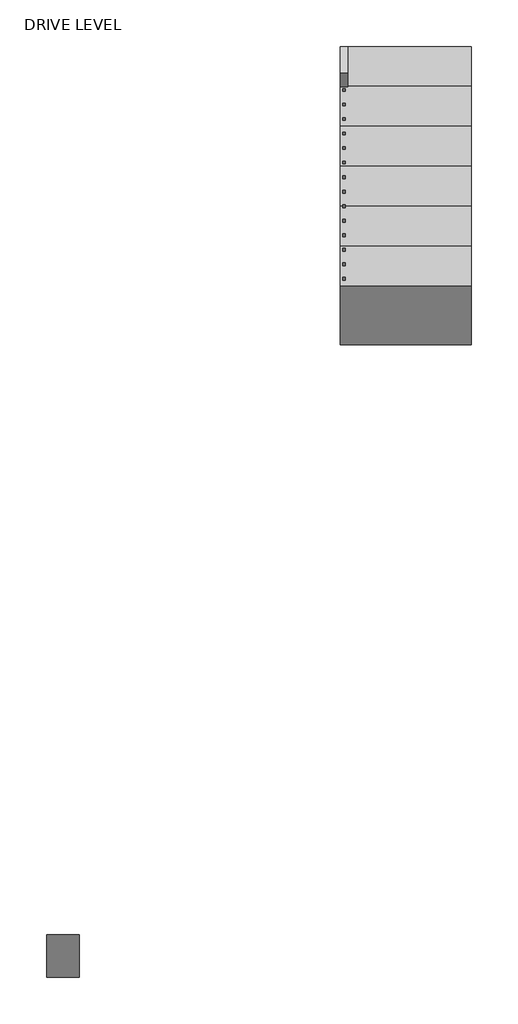
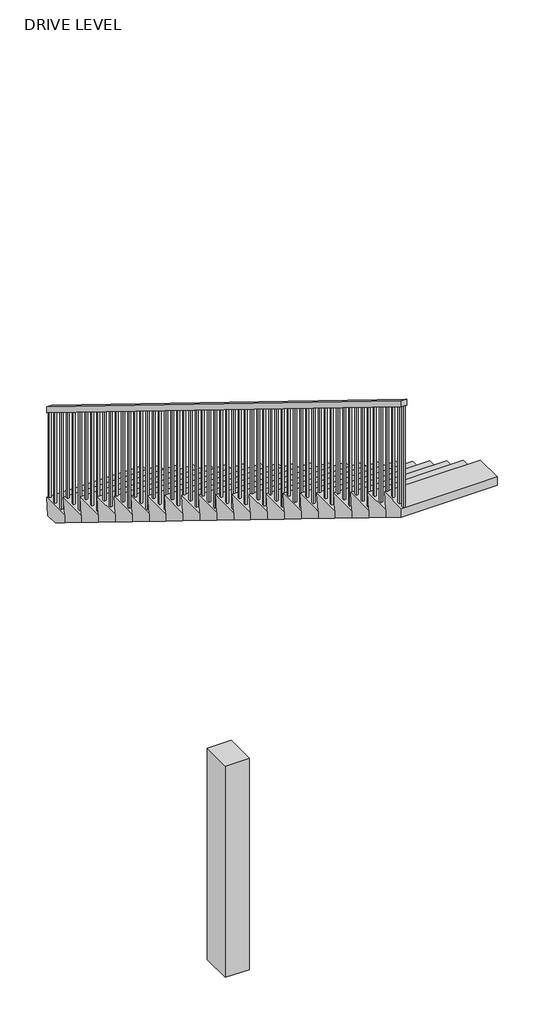
# One storey: 1 proxy, 1 railing, 1 stair flight.
"""IFC4 building model written with IfcOpenShell, lengths in millimetres."""

from ifc_helpers import new_model, si_unit, frame, origin, place, context, project, spatial, polyline, outline, extrude, faceted_brep, transform, mapped, element, save
from components import generic_models_1_generic_models_1_9fbe4478

model = new_model("IFC4")

# Units and contexts
model_context = context("Model", 3, world=origin())
ifc_project = project(units=[si_unit("LENGTHUNIT", "METRE", prefix="MILLI")], contexts=[model_context])

# Site, building, storey
site = spatial("IfcSite", under=ifc_project)
building = spatial("IfcBuilding", under=site)
storey = spatial("IfcBuildingStorey", under=building, Name="DRIVE LEVEL", Elevation=457.2)

# Proxy
placement = place(None, origin())
generic_models_1_generic_models_1_shape = generic_models_1_generic_models_1_9fbe4478(model_context)
element("IfcBuildingElementProxy", 1, Name="Generic Models 1 : Generic Models 1", ObjectType="Generic Models 1 : Generic Models 1", at=placement, inside=storey, context=model_context, shape_type="MappedRepresentation", body=[
    mapped(generic_models_1_generic_models_1_shape, transform((0.0, 0.0, 0.0), x_axis=(1.0, 0.0, 0.0), y_axis=(0.0, 1.0, 0.0), z_axis=(0.0, 0.0, 1.0))),
])

# Railing
element("IfcRailing", 2, ObjectType="Handrail - Rectangular", at=placement, inside=storey, context=model_context, shape_type="SweptSolid", body=[
    extrude(outline(polyline([(-5458.3521854, 1543.8782609), (-5458.3521854, 1484.1975237), (-11325.7521854, 5102.041002), (-11325.7521854, 5161.7217391), (-5458.3521854, 1543.8782609)])), frame((2204.5271331, 0.0, 0.0), z_axis=(1.0, 0.0, 0.0), x_axis=(0.0, 1.0, 0.0)), (0.0, 0.0, 1.0), 50.8),
    extrude(outline(polyline([(-11259.0771854, 5060.9291443), (-11240.0271854, 5049.1828992), (-11240.0271854, 4075.0434783), (-11259.0771854, 4075.0434783), (-11259.0771854, 5060.9291443)])), frame((2220.4021331, 0.0, 0.0), z_axis=(1.0, 0.0, 0.0), x_axis=(0.0, 1.0, 0.0)), (0.0, 0.0, 1.0), 19.05),
    extrude(outline(polyline([(-11157.4771854, 4998.282504), (-11138.4271854, 4986.5362589), (-11138.4271854, 4075.0434783), (-11157.4771854, 4075.0434783), (-11157.4771854, 4998.282504)])), frame((2220.4021331, 0.0, 0.0), z_axis=(1.0, 0.0, 0.0), x_axis=(0.0, 1.0, 0.0)), (0.0, 0.0, 1.0), 19.05),
    extrude(outline(polyline([(-11055.8771854, 4935.6358636), (-11036.8271854, 4923.8896186), (-11036.8271854, 4075.0434783), (-11055.8771854, 4075.0434783), (-11055.8771854, 4935.6358636)])), frame((2220.4021331, 0.0, 0.0), z_axis=(1.0, 0.0, 0.0), x_axis=(0.0, 1.0, 0.0)), (0.0, 0.0, 1.0), 19.05),
    extrude(outline(polyline([(-10954.2771854, 4872.9892233), (-10935.2271854, 4861.2429783), (-10935.2271854, 3902.7652174), (-10954.2771854, 3902.7652174), (-10954.2771854, 4872.9892233)])), frame((2220.4021331, 0.0, 0.0), z_axis=(1.0, 0.0, 0.0), x_axis=(0.0, 1.0, 0.0)), (0.0, 0.0, 1.0), 19.05),
    extrude(outline(polyline([(-10852.6771854, 4810.342583), (-10833.6271854, 4798.596338), (-10833.6271854, 3902.7652174), (-10852.6771854, 3902.7652174), (-10852.6771854, 4810.342583)])), frame((2220.4021331, 0.0, 0.0), z_axis=(1.0, 0.0, 0.0), x_axis=(0.0, 1.0, 0.0)), (0.0, 0.0, 1.0), 19.05),
    extrude(outline(polyline([(-10751.0771854, 4747.6959427), (-10732.0271854, 4735.9496976), (-10732.0271854, 3730.4869565), (-10751.0771854, 3730.4869565), (-10751.0771854, 4747.6959427)])), frame((2220.4021331, 0.0, 0.0), z_axis=(1.0, 0.0, 0.0), x_axis=(0.0, 1.0, 0.0)), (0.0, 0.0, 1.0), 19.05),
    extrude(outline(polyline([(-10649.4771854, 4685.0493024), (-10630.4271854, 4673.3030573), (-10630.4271854, 3730.4869565), (-10649.4771854, 3730.4869565), (-10649.4771854, 4685.0493024)])), frame((2220.4021331, 0.0, 0.0), z_axis=(1.0, 0.0, 0.0), x_axis=(0.0, 1.0, 0.0)), (0.0, 0.0, 1.0), 19.05),
    extrude(outline(polyline([(-10547.8771854, 4622.4026621), (-10528.8271854, 4610.656417), (-10528.8271854, 3730.4869565), (-10547.8771854, 3730.4869565), (-10547.8771854, 4622.4026621)])), frame((2220.4021331, 0.0, 0.0), z_axis=(1.0, 0.0, 0.0), x_axis=(0.0, 1.0, 0.0)), (0.0, 0.0, 1.0), 19.05),
    extrude(outline(polyline([(-10446.2771854, 4559.7560218), (-10427.2271854, 4548.0097767), (-10427.2271854, 3558.2086957), (-10446.2771854, 3558.2086957), (-10446.2771854, 4559.7560218)])), frame((2220.4021331, 0.0, 0.0), z_axis=(1.0, 0.0, 0.0), x_axis=(0.0, 1.0, 0.0)), (0.0, 0.0, 1.0), 19.05),
    extrude(outline(polyline([(-10344.6771854, 4497.1093814), (-10325.6271854, 4485.3631364), (-10325.6271854, 3558.2086957), (-10344.6771854, 3558.2086957), (-10344.6771854, 4497.1093814)])), frame((2220.4021331, 0.0, 0.0), z_axis=(1.0, 0.0, 0.0), x_axis=(0.0, 1.0, 0.0)), (0.0, 0.0, 1.0), 19.05),
    extrude(outline(polyline([(-10243.0771854, 4434.4627411), (-10224.0271854, 4422.7164961), (-10224.0271854, 3558.2086957), (-10243.0771854, 3558.2086957), (-10243.0771854, 4434.4627411)])), frame((2220.4021331, 0.0, 0.0), z_axis=(1.0, 0.0, 0.0), x_axis=(0.0, 1.0, 0.0)), (0.0, 0.0, 1.0), 19.05),
    extrude(outline(polyline([(-10141.4771854, 4371.8161008), (-10122.4271854, 4360.0698557), (-10122.4271854, 3385.9304348), (-10141.4771854, 3385.9304348), (-10141.4771854, 4371.8161008)])), frame((2220.4021331, 0.0, 0.0), z_axis=(1.0, 0.0, 0.0), x_axis=(0.0, 1.0, 0.0)), (0.0, 0.0, 1.0), 19.05),
    extrude(outline(polyline([(-10039.8771854, 4309.1694605), (-10020.8271854, 4297.4232154), (-10020.8271854, 3385.9304348), (-10039.8771854, 3385.9304348), (-10039.8771854, 4309.1694605)])), frame((2220.4021331, 0.0, 0.0), z_axis=(1.0, 0.0, 0.0), x_axis=(0.0, 1.0, 0.0)), (0.0, 0.0, 1.0), 19.05),
    extrude(outline(polyline([(-9938.2771854, 4246.5228202), (-9919.2271854, 4234.7765751), (-9919.2271854, 3385.9304348), (-9938.2771854, 3385.9304348), (-9938.2771854, 4246.5228202)])), frame((2220.4021331, 0.0, 0.0), z_axis=(1.0, 0.0, 0.0), x_axis=(0.0, 1.0, 0.0)), (0.0, 0.0, 1.0), 19.05),
    extrude(outline(polyline([(-9836.6771854, 4183.8761799), (-9817.6271854, 4172.1299348), (-9817.6271854, 3213.6521739), (-9836.6771854, 3213.6521739), (-9836.6771854, 4183.8761799)])), frame((2220.4021331, 0.0, 0.0), z_axis=(1.0, 0.0, 0.0), x_axis=(0.0, 1.0, 0.0)), (0.0, 0.0, 1.0), 19.05),
    extrude(outline(polyline([(-9735.0771854, 4121.2295395), (-9716.0271854, 4109.4832945), (-9716.0271854, 3213.6521739), (-9735.0771854, 3213.6521739), (-9735.0771854, 4121.2295395)])), frame((2220.4021331, 0.0, 0.0), z_axis=(1.0, 0.0, 0.0), x_axis=(0.0, 1.0, 0.0)), (0.0, 0.0, 1.0), 19.05),
    extrude(outline(polyline([(-9633.4771854, 4058.5828992), (-9614.4271854, 4046.8366542), (-9614.4271854, 3041.373913), (-9633.4771854, 3041.373913), (-9633.4771854, 4058.5828992)])), frame((2220.4021331, 0.0, 0.0), z_axis=(1.0, 0.0, 0.0), x_axis=(0.0, 1.0, 0.0)), (0.0, 0.0, 1.0), 19.05),
    extrude(outline(polyline([(-9531.8771854, 3995.9362589), (-9512.8271854, 3984.1900138), (-9512.8271854, 3041.373913), (-9531.8771854, 3041.373913), (-9531.8771854, 3995.9362589)])), frame((2220.4021331, 0.0, 0.0), z_axis=(1.0, 0.0, 0.0), x_axis=(0.0, 1.0, 0.0)), (0.0, 0.0, 1.0), 19.05),
    extrude(outline(polyline([(-9430.2771854, 3933.2896186), (-9411.2271854, 3921.5433735), (-9411.2271854, 3041.373913), (-9430.2771854, 3041.373913), (-9430.2771854, 3933.2896186)])), frame((2220.4021331, 0.0, 0.0), z_axis=(1.0, 0.0, 0.0), x_axis=(0.0, 1.0, 0.0)), (0.0, 0.0, 1.0), 19.05),
    extrude(outline(polyline([(-9328.6771854, 3870.6429783), (-9309.6271854, 3858.8967332), (-9309.6271854, 2869.0956522), (-9328.6771854, 2869.0956522), (-9328.6771854, 3870.6429783)])), frame((2220.4021331, 0.0, 0.0), z_axis=(1.0, 0.0, 0.0), x_axis=(0.0, 1.0, 0.0)), (0.0, 0.0, 1.0), 19.05),
    extrude(outline(polyline([(-9227.0771854, 3807.996338), (-9208.0271854, 3796.2500929), (-9208.0271854, 2869.0956522), (-9227.0771854, 2869.0956522), (-9227.0771854, 3807.996338)])), frame((2220.4021331, 0.0, 0.0), z_axis=(1.0, 0.0, 0.0), x_axis=(0.0, 1.0, 0.0)), (0.0, 0.0, 1.0), 19.05),
    extrude(outline(polyline([(-9125.4771854, 3745.3496976), (-9106.4271854, 3733.6034526), (-9106.4271854, 2869.0956522), (-9125.4771854, 2869.0956522), (-9125.4771854, 3745.3496976)])), frame((2220.4021331, 0.0, 0.0), z_axis=(1.0, 0.0, 0.0), x_axis=(0.0, 1.0, 0.0)), (0.0, 0.0, 1.0), 19.05),
    extrude(outline(polyline([(-9023.8771854, 3682.7030573), (-9004.8271854, 3670.9568123), (-9004.8271854, 2696.8173913), (-9023.8771854, 2696.8173913), (-9023.8771854, 3682.7030573)])), frame((2220.4021331, 0.0, 0.0), z_axis=(1.0, 0.0, 0.0), x_axis=(0.0, 1.0, 0.0)), (0.0, 0.0, 1.0), 19.05),
    extrude(outline(polyline([(-8922.2771854, 3620.056417), (-8903.2271854, 3608.3101719), (-8903.2271854, 2696.8173913), (-8922.2771854, 2696.8173913), (-8922.2771854, 3620.056417)])), frame((2220.4021331, 0.0, 0.0), z_axis=(1.0, 0.0, 0.0), x_axis=(0.0, 1.0, 0.0)), (0.0, 0.0, 1.0), 19.05),
    extrude(outline(polyline([(-8820.6771854, 3557.4097767), (-8801.6271854, 3545.6635316), (-8801.6271854, 2696.8173913), (-8820.6771854, 2696.8173913), (-8820.6771854, 3557.4097767)])), frame((2220.4021331, 0.0, 0.0), z_axis=(1.0, 0.0, 0.0), x_axis=(0.0, 1.0, 0.0)), (0.0, 0.0, 1.0), 19.05),
    extrude(outline(polyline([(-8719.0771854, 3494.7631364), (-8700.0271854, 3483.0168913), (-8700.0271854, 2524.5391304), (-8719.0771854, 2524.5391304), (-8719.0771854, 3494.7631364)])), frame((2220.4021331, 0.0, 0.0), z_axis=(1.0, 0.0, 0.0), x_axis=(0.0, 1.0, 0.0)), (0.0, 0.0, 1.0), 19.05),
    extrude(outline(polyline([(-8617.4771854, 3432.1164961), (-8598.4271854, 3420.370251), (-8598.4271854, 2524.5391304), (-8617.4771854, 2524.5391304), (-8617.4771854, 3432.1164961)])), frame((2220.4021331, 0.0, 0.0), z_axis=(1.0, 0.0, 0.0), x_axis=(0.0, 1.0, 0.0)), (0.0, 0.0, 1.0), 19.05),
    extrude(outline(polyline([(-8515.8771854, 3369.4698557), (-8496.8271854, 3357.7236107), (-8496.8271854, 2352.2608696), (-8515.8771854, 2352.2608696), (-8515.8771854, 3369.4698557)])), frame((2220.4021331, 0.0, 0.0), z_axis=(1.0, 0.0, 0.0), x_axis=(0.0, 1.0, 0.0)), (0.0, 0.0, 1.0), 19.05),
    extrude(outline(polyline([(-8414.2771854, 3306.8232154), (-8395.2271854, 3295.0769704), (-8395.2271854, 2352.2608696), (-8414.2771854, 2352.2608696), (-8414.2771854, 3306.8232154)])), frame((2220.4021331, 0.0, 0.0), z_axis=(1.0, 0.0, 0.0), x_axis=(0.0, 1.0, 0.0)), (0.0, 0.0, 1.0), 19.05),
    extrude(outline(polyline([(-8312.6771854, 3244.1765751), (-8293.6271854, 3232.4303301), (-8293.6271854, 2352.2608696), (-8312.6771854, 2352.2608696), (-8312.6771854, 3244.1765751)])), frame((2220.4021331, 0.0, 0.0), z_axis=(1.0, 0.0, 0.0), x_axis=(0.0, 1.0, 0.0)), (0.0, 0.0, 1.0), 19.05),
    extrude(outline(polyline([(-8211.0771854, 3181.5299348), (-8192.0271854, 3169.7836897), (-8192.0271854, 2179.9826087), (-8211.0771854, 2179.9826087), (-8211.0771854, 3181.5299348)])), frame((2220.4021331, 0.0, 0.0), z_axis=(1.0, 0.0, 0.0), x_axis=(0.0, 1.0, 0.0)), (0.0, 0.0, 1.0), 19.05),
    extrude(outline(polyline([(-8109.4771854, 3118.8832945), (-8090.4271854, 3107.1370494), (-8090.4271854, 2179.9826087), (-8109.4771854, 2179.9826087), (-8109.4771854, 3118.8832945)])), frame((2220.4021331, 0.0, 0.0), z_axis=(1.0, 0.0, 0.0), x_axis=(0.0, 1.0, 0.0)), (0.0, 0.0, 1.0), 19.05),
    extrude(outline(polyline([(-8007.8771854, 3056.2366542), (-7988.8271854, 3044.4904091), (-7988.8271854, 2179.9826087), (-8007.8771854, 2179.9826087), (-8007.8771854, 3056.2366542)])), frame((2220.4021331, 0.0, 0.0), z_axis=(1.0, 0.0, 0.0), x_axis=(0.0, 1.0, 0.0)), (0.0, 0.0, 1.0), 19.05),
    extrude(outline(polyline([(-7906.2771854, 2993.5900138), (-7887.2271854, 2981.8437688), (-7887.2271854, 2007.7043478), (-7906.2771854, 2007.7043478), (-7906.2771854, 2993.5900138)])), frame((2220.4021331, 0.0, 0.0), z_axis=(1.0, 0.0, 0.0), x_axis=(0.0, 1.0, 0.0)), (0.0, 0.0, 1.0), 19.05),
    extrude(outline(polyline([(-7804.6771854, 2930.9433735), (-7785.6271854, 2919.1971285), (-7785.6271854, 2007.7043478), (-7804.6771854, 2007.7043478), (-7804.6771854, 2930.9433735)])), frame((2220.4021331, 0.0, 0.0), z_axis=(1.0, 0.0, 0.0), x_axis=(0.0, 1.0, 0.0)), (0.0, 0.0, 1.0), 19.05),
    extrude(outline(polyline([(-7703.0771854, 2868.2967332), (-7684.0271854, 2856.5504882), (-7684.0271854, 2007.7043478), (-7703.0771854, 2007.7043478), (-7703.0771854, 2868.2967332)])), frame((2220.4021331, 0.0, 0.0), z_axis=(1.0, 0.0, 0.0), x_axis=(0.0, 1.0, 0.0)), (0.0, 0.0, 1.0), 19.05),
    extrude(outline(polyline([(-7601.4771854, 2805.6500929), (-7582.4271854, 2793.9038478), (-7582.4271854, 1835.426087), (-7601.4771854, 1835.426087), (-7601.4771854, 2805.6500929)])), frame((2220.4021331, 0.0, 0.0), z_axis=(1.0, 0.0, 0.0), x_axis=(0.0, 1.0, 0.0)), (0.0, 0.0, 1.0), 19.05),
    extrude(outline(polyline([(-7499.8771854, 2743.0034526), (-7480.8271854, 2731.2572075), (-7480.8271854, 1835.426087), (-7499.8771854, 1835.426087), (-7499.8771854, 2743.0034526)])), frame((2220.4021331, 0.0, 0.0), z_axis=(1.0, 0.0, 0.0), x_axis=(0.0, 1.0, 0.0)), (0.0, 0.0, 1.0), 19.05),
    extrude(outline(polyline([(-7398.2771854, 2680.3568123), (-7379.2271854, 2668.6105672), (-7379.2271854, 1663.1478261), (-7398.2771854, 1663.1478261), (-7398.2771854, 2680.3568123)])), frame((2220.4021331, 0.0, 0.0), z_axis=(1.0, 0.0, 0.0), x_axis=(0.0, 1.0, 0.0)), (0.0, 0.0, 1.0), 19.05),
    extrude(outline(polyline([(-7296.6771854, 2617.7101719), (-7277.6271854, 2605.9639269), (-7277.6271854, 1663.1478261), (-7296.6771854, 1663.1478261), (-7296.6771854, 2617.7101719)])), frame((2220.4021331, 0.0, 0.0), z_axis=(1.0, 0.0, 0.0), x_axis=(0.0, 1.0, 0.0)), (0.0, 0.0, 1.0), 19.05),
    extrude(outline(polyline([(-7195.0771854, 2555.0635316), (-7176.0271854, 2543.3172866), (-7176.0271854, 1663.1478261), (-7195.0771854, 1663.1478261), (-7195.0771854, 2555.0635316)])), frame((2220.4021331, 0.0, 0.0), z_axis=(1.0, 0.0, 0.0), x_axis=(0.0, 1.0, 0.0)), (0.0, 0.0, 1.0), 19.05),
    extrude(outline(polyline([(-7093.4771854, 2492.4168913), (-7074.4271854, 2480.6706463), (-7074.4271854, 1490.8695652), (-7093.4771854, 1490.8695652), (-7093.4771854, 2492.4168913)])), frame((2220.4021331, 0.0, 0.0), z_axis=(1.0, 0.0, 0.0), x_axis=(0.0, 1.0, 0.0)), (0.0, 0.0, 1.0), 19.05),
    extrude(outline(polyline([(-6991.8771854, 2429.770251), (-6972.8271854, 2418.0240059), (-6972.8271854, 1490.8695652), (-6991.8771854, 1490.8695652), (-6991.8771854, 2429.770251)])), frame((2220.4021331, 0.0, 0.0), z_axis=(1.0, 0.0, 0.0), x_axis=(0.0, 1.0, 0.0)), (0.0, 0.0, 1.0), 19.05),
    extrude(outline(polyline([(-6890.2771854, 2367.1236107), (-6871.2271854, 2355.3773656), (-6871.2271854, 1490.8695652), (-6890.2771854, 1490.8695652), (-6890.2771854, 2367.1236107)])), frame((2220.4021331, 0.0, 0.0), z_axis=(1.0, 0.0, 0.0), x_axis=(0.0, 1.0, 0.0)), (0.0, 0.0, 1.0), 19.05),
    extrude(outline(polyline([(-6788.6771854, 2304.4769704), (-6769.6271854, 2292.7307253), (-6769.6271854, 1318.5913043), (-6788.6771854, 1318.5913043), (-6788.6771854, 2304.4769704)])), frame((2220.4021331, 0.0, 0.0), z_axis=(1.0, 0.0, 0.0), x_axis=(0.0, 1.0, 0.0)), (0.0, 0.0, 1.0), 19.05),
    extrude(outline(polyline([(-6687.0771854, 2241.8303301), (-6668.0271854, 2230.084085), (-6668.0271854, 1318.5913043), (-6687.0771854, 1318.5913043), (-6687.0771854, 2241.8303301)])), frame((2220.4021331, 0.0, 0.0), z_axis=(1.0, 0.0, 0.0), x_axis=(0.0, 1.0, 0.0)), (0.0, 0.0, 1.0), 19.05),
    extrude(outline(polyline([(-6585.4771854, 2179.1836897), (-6566.4271854, 2167.4374447), (-6566.4271854, 1318.5913043), (-6585.4771854, 1318.5913043), (-6585.4771854, 2179.1836897)])), frame((2220.4021331, 0.0, 0.0), z_axis=(1.0, 0.0, 0.0), x_axis=(0.0, 1.0, 0.0)), (0.0, 0.0, 1.0), 19.05),
    extrude(outline(polyline([(-6483.8771854, 2116.5370494), (-6464.8271854, 2104.7908044), (-6464.8271854, 1146.3130435), (-6483.8771854, 1146.3130435), (-6483.8771854, 2116.5370494)])), frame((2220.4021331, 0.0, 0.0), z_axis=(1.0, 0.0, 0.0), x_axis=(0.0, 1.0, 0.0)), (0.0, 0.0, 1.0), 19.05),
    extrude(outline(polyline([(-6382.2771854, 2053.8904091), (-6363.2271854, 2042.144164), (-6363.2271854, 1146.3130435), (-6382.2771854, 1146.3130435), (-6382.2771854, 2053.8904091)])), frame((2220.4021331, 0.0, 0.0), z_axis=(1.0, 0.0, 0.0), x_axis=(0.0, 1.0, 0.0)), (0.0, 0.0, 1.0), 19.05),
    extrude(outline(polyline([(-6280.6771854, 1991.2437688), (-6261.6271854, 1979.4975237), (-6261.6271854, 974.0347826), (-6280.6771854, 974.0347826), (-6280.6771854, 1991.2437688)])), frame((2220.4021331, 0.0, 0.0), z_axis=(1.0, 0.0, 0.0), x_axis=(0.0, 1.0, 0.0)), (0.0, 0.0, 1.0), 19.05),
    extrude(outline(polyline([(-6179.0771854, 1928.5971285), (-6160.0271854, 1916.8508834), (-6160.0271854, 974.0347826), (-6179.0771854, 974.0347826), (-6179.0771854, 1928.5971285)])), frame((2220.4021331, 0.0, 0.0), z_axis=(1.0, 0.0, 0.0), x_axis=(0.0, 1.0, 0.0)), (0.0, 0.0, 1.0), 19.05),
    extrude(outline(polyline([(-6077.4771854, 1865.9504882), (-6058.4271854, 1854.2042431), (-6058.4271854, 974.0347826), (-6077.4771854, 974.0347826), (-6077.4771854, 1865.9504882)])), frame((2220.4021331, 0.0, 0.0), z_axis=(1.0, 0.0, 0.0), x_axis=(0.0, 1.0, 0.0)), (0.0, 0.0, 1.0), 19.05),
    extrude(outline(polyline([(-5975.8771854, 1803.3038478), (-5956.8271854, 1791.5576028), (-5956.8271854, 801.7565217), (-5975.8771854, 801.7565217), (-5975.8771854, 1803.3038478)])), frame((2220.4021331, 0.0, 0.0), z_axis=(1.0, 0.0, 0.0), x_axis=(0.0, 1.0, 0.0)), (0.0, 0.0, 1.0), 19.05),
    extrude(outline(polyline([(-5874.2771854, 1740.6572075), (-5855.2271854, 1728.9109625), (-5855.2271854, 801.7565217), (-5874.2771854, 801.7565217), (-5874.2771854, 1740.6572075)])), frame((2220.4021331, 0.0, 0.0), z_axis=(1.0, 0.0, 0.0), x_axis=(0.0, 1.0, 0.0)), (0.0, 0.0, 1.0), 19.05),
    extrude(outline(polyline([(-5772.6771854, 1678.0105672), (-5753.6271854, 1666.2643221), (-5753.6271854, 801.7565217), (-5772.6771854, 801.7565217), (-5772.6771854, 1678.0105672)])), frame((2220.4021331, 0.0, 0.0), z_axis=(1.0, 0.0, 0.0), x_axis=(0.0, 1.0, 0.0)), (0.0, 0.0, 1.0), 19.05),
    extrude(outline(polyline([(-5671.0771854, 1615.3639269), (-5652.0271854, 1603.6176818), (-5652.0271854, 629.4782609), (-5671.0771854, 629.4782609), (-5671.0771854, 1615.3639269)])), frame((2220.4021331, 0.0, 0.0), z_axis=(1.0, 0.0, 0.0), x_axis=(0.0, 1.0, 0.0)), (0.0, 0.0, 1.0), 19.05),
    extrude(outline(polyline([(-5569.4771854, 1552.7172866), (-5550.4271854, 1540.9710415), (-5550.4271854, 629.4782609), (-5569.4771854, 629.4782609), (-5569.4771854, 1552.7172866)])), frame((2220.4021331, 0.0, 0.0), z_axis=(1.0, 0.0, 0.0), x_axis=(0.0, 1.0, 0.0)), (0.0, 0.0, 1.0), 19.05),
    extrude(outline(polyline([(-11325.7521854, 5102.041002), (-11306.7021854, 5090.2947569), (-11306.7021854, 4075.0434783), (-11325.7521854, 4075.0434783), (-11325.7521854, 5102.041002)])), frame((2220.4021331, 0.0, 0.0), z_axis=(1.0, 0.0, 0.0), x_axis=(0.0, 1.0, 0.0)), (0.0, 0.0, 1.0), 19.05),
    extrude(outline(polyline([(-5477.4021854, 1495.9437688), (-5458.3521854, 1484.1975237), (-5458.3521854, 629.4782609), (-5477.4021854, 629.4782609), (-5477.4021854, 1495.9437688)])), frame((2220.4021331, 0.0, 0.0), z_axis=(1.0, 0.0, 0.0), x_axis=(0.0, 1.0, 0.0)), (0.0, 0.0, 1.0), 19.05),
])

# Stair flight
element("IfcStairFlight", 3, ObjectType="3/4\" Nosing", at=placement, inside=storey, context=model_context, shape_type="Brep", body=[
    faceted_brep([(3118.9271331, -5458.3521854, 629.4782609), (2204.5271331, -5458.3521854, 629.4782609), (2204.5271331, -5756.8021854, 629.4782609), (3118.9271331, -5756.8021854, 629.4782609), (3118.9271331, -5756.8021854, 554.8773394), (3118.9271331, -5598.3895772, 457.2), (3118.9271331, -5477.4021854, 457.2), (2204.5271331, -5477.4021854, 457.2), (2204.5271331, -5598.3895772, 457.2), (2204.5271331, -5756.8021854, 554.8773394), (3118.9271331, -5737.7521854, 801.7565217), (2204.5271331, -5737.7521854, 801.7565217), (2204.5271331, -6036.2021854, 801.7565217), (3118.9271331, -6036.2021854, 801.7565217), (3118.9271331, -6036.2021854, 727.1556003), (2204.5271331, -6036.2021854, 727.1556003), (3118.9271331, -6017.1521854, 974.0347826), (2204.5271331, -6017.1521854, 974.0347826), (2204.5271331, -6315.6021854, 974.0347826), (3118.9271331, -6315.6021854, 974.0347826), (3118.9271331, -6315.6021854, 899.4338612), (2204.5271331, -6315.6021854, 899.4338612), (3118.9271331, -6296.5521854, 1146.3130435), (2204.5271331, -6296.5521854, 1146.3130435), (2204.5271331, -6595.0021854, 1146.3130435), (3118.9271331, -6595.0021854, 1146.3130435), (3118.9271331, -6595.0021854, 1071.7121221), (2204.5271331, -6595.0021854, 1071.7121221), (3118.9271331, -6575.9521854, 1318.5913043), (2204.5271331, -6575.9521854, 1318.5913043), (2204.5271331, -6874.4021854, 1318.5913043), (3118.9271331, -6874.4021854, 1318.5913043), (3118.9271331, -6874.4021854, 1243.9903829), (2204.5271331, -6874.4021854, 1243.9903829), (3118.9271331, -6855.3521854, 1490.8695652), (2204.5271331, -6855.3521854, 1490.8695652), (2204.5271331, -7153.8021854, 1490.8695652), (3118.9271331, -7153.8021854, 1490.8695652), (3118.9271331, -7153.8021854, 1416.2686438), (2204.5271331, -7153.8021854, 1416.2686438), (3118.9271331, -7134.7521854, 1663.1478261), (2204.5271331, -7134.7521854, 1663.1478261), (2204.5271331, -7433.2021854, 1663.1478261), (3118.9271331, -7433.2021854, 1663.1478261), (3118.9271331, -7433.2021854, 1588.5469047), (2204.5271331, -7433.2021854, 1588.5469047), (3118.9271331, -7414.1521854, 1835.426087), (2204.5271331, -7414.1521854, 1835.426087), (2204.5271331, -7712.6021854, 1835.426087), (3118.9271331, -7712.6021854, 1835.426087), (3118.9271331, -7712.6021854, 1760.8251655), (2204.5271331, -7712.6021854, 1760.8251655), (3118.9271331, -7693.5521854, 2007.7043478), (2204.5271331, -7693.5521854, 2007.7043478), (2204.5271331, -7992.0021854, 2007.7043478), (3118.9271331, -7992.0021854, 2007.7043478), (3118.9271331, -7992.0021854, 1933.1034264), (2204.5271331, -7992.0021854, 1933.1034264), (3118.9271331, -7972.9521854, 2179.9826087), (2204.5271331, -7972.9521854, 2179.9826087), (2204.5271331, -8271.4021854, 2179.9826087), (3118.9271331, -8271.4021854, 2179.9826087), (3118.9271331, -8271.4021854, 2105.3816873), (2204.5271331, -8271.4021854, 2105.3816873), (3118.9271331, -8252.3521854, 2352.2608696), (2204.5271331, -8252.3521854, 2352.2608696), (2204.5271331, -8550.8021854, 2352.2608696), (3118.9271331, -8550.8021854, 2352.2608696), (3118.9271331, -8550.8021854, 2277.6599481), (2204.5271331, -8550.8021854, 2277.6599481), (3118.9271331, -8830.2021854, 2449.938209), (3118.9271331, -9109.6021854, 2622.2164699), (3118.9271331, -9389.0021854, 2794.4947307), (3118.9271331, -9668.4021854, 2966.7729916), (3118.9271331, -9947.8021854, 3139.0512525), (3118.9271331, -10227.2021854, 3311.3295134), (3118.9271331, -10506.6021854, 3483.6077742), (3118.9271331, -10786.0021854, 3655.8860351), (3118.9271331, -11065.4021854, 3828.164296), (3118.9271331, -11325.7521854, 3988.6963118), (2204.5271331, -11325.7521854, 3988.6963118), (2204.5271331, -11065.4021854, 3828.164296), (2204.5271331, -10786.0021854, 3655.8860351), (2204.5271331, -10506.6021854, 3483.6077742), (2204.5271331, -10227.2021854, 3311.3295134), (2204.5271331, -9947.8021854, 3139.0512525), (2204.5271331, -9668.4021854, 2966.7729916), (2204.5271331, -9389.0021854, 2794.4947307), (2204.5271331, -9109.6021854, 2622.2164699), (2204.5271331, -8830.2021854, 2449.938209), (3118.9271331, -8531.7521854, 2524.5391304), (2204.5271331, -8531.7521854, 2524.5391304), (2204.5271331, -8830.2021854, 2524.5391304), (3118.9271331, -8830.2021854, 2524.5391304), (3118.9271331, -8811.1521854, 2696.8173913), (2204.5271331, -8811.1521854, 2696.8173913), (2204.5271331, -9109.6021854, 2696.8173913), (3118.9271331, -9109.6021854, 2696.8173913), (3118.9271331, -9090.5521854, 2869.0956522), (2204.5271331, -9090.5521854, 2869.0956522), (2204.5271331, -9389.0021854, 2869.0956522), (3118.9271331, -9389.0021854, 2869.0956522), (3118.9271331, -9369.9521854, 3041.373913), (2204.5271331, -9369.9521854, 3041.373913), (2204.5271331, -9668.4021854, 3041.373913), (3118.9271331, -9668.4021854, 3041.373913), (3118.9271331, -9649.3521854, 3213.6521739), (2204.5271331, -9649.3521854, 3213.6521739), (2204.5271331, -9947.8021854, 3213.6521739), (3118.9271331, -9947.8021854, 3213.6521739), (3118.9271331, -9928.7521854, 3385.9304348), (2204.5271331, -9928.7521854, 3385.9304348), (2204.5271331, -10227.2021854, 3385.9304348), (3118.9271331, -10227.2021854, 3385.9304348), (3118.9271331, -10208.1521854, 3558.2086957), (2204.5271331, -10208.1521854, 3558.2086957), (2204.5271331, -10506.6021854, 3558.2086957), (3118.9271331, -10506.6021854, 3558.2086957), (3118.9271331, -10487.5521854, 3730.4869565), (2204.5271331, -10487.5521854, 3730.4869565), (2204.5271331, -10786.0021854, 3730.4869565), (3118.9271331, -10786.0021854, 3730.4869565), (3118.9271331, -10766.9521854, 3902.7652174), (2204.5271331, -10766.9521854, 3902.7652174), (2204.5271331, -11065.4021854, 3902.7652174), (3118.9271331, -11065.4021854, 3902.7652174), (3118.9271331, -11046.3521854, 4075.0434783), (2204.5271331, -11046.3521854, 4075.0434783), (2204.5271331, -11325.7521854, 4075.0434783), (3118.9271331, -11325.7521854, 4075.0434783)], [[[0, 1, 2, 3]], [[0, 3, 4, 5, 6]], [[2, 1, 7, 8, 9]], [[10, 11, 12, 13]], [[10, 13, 14, 4, 3]], [[12, 11, 2, 9, 15]], [[16, 17, 18, 19]], [[16, 19, 20, 14, 13]], [[18, 17, 12, 15, 21]], [[22, 23, 24, 25]], [[22, 25, 26, 20, 19]], [[24, 23, 18, 21, 27]], [[28, 29, 30, 31]], [[28, 31, 32, 26, 25]], [[30, 29, 24, 27, 33]], [[34, 35, 36, 37]], [[34, 37, 38, 32, 31]], [[36, 35, 30, 33, 39]], [[40, 41, 42, 43]], [[40, 43, 44, 38, 37]], [[42, 41, 36, 39, 45]], [[46, 47, 48, 49]], [[46, 49, 50, 44, 43]], [[48, 47, 42, 45, 51]], [[52, 53, 54, 55]], [[52, 55, 56, 50, 49]], [[54, 53, 48, 51, 57]], [[58, 59, 60, 61]], [[58, 61, 62, 56, 55]], [[60, 59, 54, 57, 63]], [[64, 65, 66, 67]], [[64, 67, 68, 62, 61]], [[66, 65, 60, 63, 69]], [[1, 0, 6, 7]], [[3, 2, 11, 10]], [[13, 12, 17, 16]], [[19, 18, 23, 22]], [[25, 24, 29, 28]], [[31, 30, 35, 34]], [[37, 36, 41, 40]], [[43, 42, 47, 46]], [[49, 48, 53, 52]], [[55, 54, 59, 58]], [[7, 6, 5, 8]], [[8, 5, 4, 14, 20, 26, 32, 38, 44, 50, 56, 62, 68, 70, 71, 72, 73, 74, 75, 76, 77, 78, 79, 80, 81, 82, 83, 84, 85, 86, 87, 88, 89, 69, 63, 57, 51, 45, 39, 33, 27, 21, 15, 9]], [[61, 60, 65, 64]], [[90, 91, 92, 93]], [[90, 93, 70, 68, 67]], [[92, 91, 66, 69, 89]], [[67, 66, 91, 90]], [[94, 95, 96, 97]], [[94, 97, 71, 70, 93]], [[96, 95, 92, 89, 88]], [[93, 92, 95, 94]], [[98, 99, 100, 101]], [[98, 101, 72, 71, 97]], [[100, 99, 96, 88, 87]], [[97, 96, 99, 98]], [[102, 103, 104, 105]], [[102, 105, 73, 72, 101]], [[104, 103, 100, 87, 86]], [[101, 100, 103, 102]], [[106, 107, 108, 109]], [[106, 109, 74, 73, 105]], [[108, 107, 104, 86, 85]], [[105, 104, 107, 106]], [[110, 111, 112, 113]], [[110, 113, 75, 74, 109]], [[112, 111, 108, 85, 84]], [[109, 108, 111, 110]], [[114, 115, 116, 117]], [[114, 117, 76, 75, 113]], [[116, 115, 112, 84, 83]], [[113, 112, 115, 114]], [[118, 119, 120, 121]], [[118, 121, 77, 76, 117]], [[120, 119, 116, 83, 82]], [[117, 116, 119, 118]], [[122, 123, 124, 125]], [[122, 125, 78, 77, 121]], [[124, 123, 120, 82, 81]], [[121, 120, 123, 122]], [[126, 127, 128, 129]], [[126, 129, 79, 78, 125]], [[128, 127, 124, 81, 80]], [[129, 128, 80, 79]], [[125, 124, 127, 126]]]),
])

save(model, "model.ifc")

# Revit data of these elements
# Type "Handrail - Rectangular"
#   Assembly Code = "C2010400"
#   built-in parameter 1008612 = 0.0416667 (stored number, unit not read)
#   built-in parameter 1008611 = 0.0416667 (stored number, unit not read)
#   built-in parameter 1008609 = 0.333333 (stored number, unit not read)
#   built-in parameter 1008604 = 0.166667 (stored number, unit not read)
#   built-in parameter 1008603 = 0.166667 (stored number, unit not read)
#   Railing Height = 3' - 0"
#   built-in parameter 1008630 = 2
#   built-in parameter 1008610 = 2
#   built-in parameter 1008618 = Baluster - Square : 3/4"
# Element 1 (IfcBuildingElementProxy, "Generic Models 1 : Generic Models 1")
#   Phase Created = New Construction
# Element 2 (IfcRailing, "Handrail - Rectangular")
#   Phase Created = New Construction
# Element 3 (IfcStairFlight, "3/4\" Nosing")
#   Phase Created = New Construction
#   Materials on its faces: "Gypsum Wall Board"
# Materials
#   "Gypsum Wall Board": class "Generic", colour RGB 228 228 228, transparency 0, Description = "Gypsum Wall Board", Cost = 0
